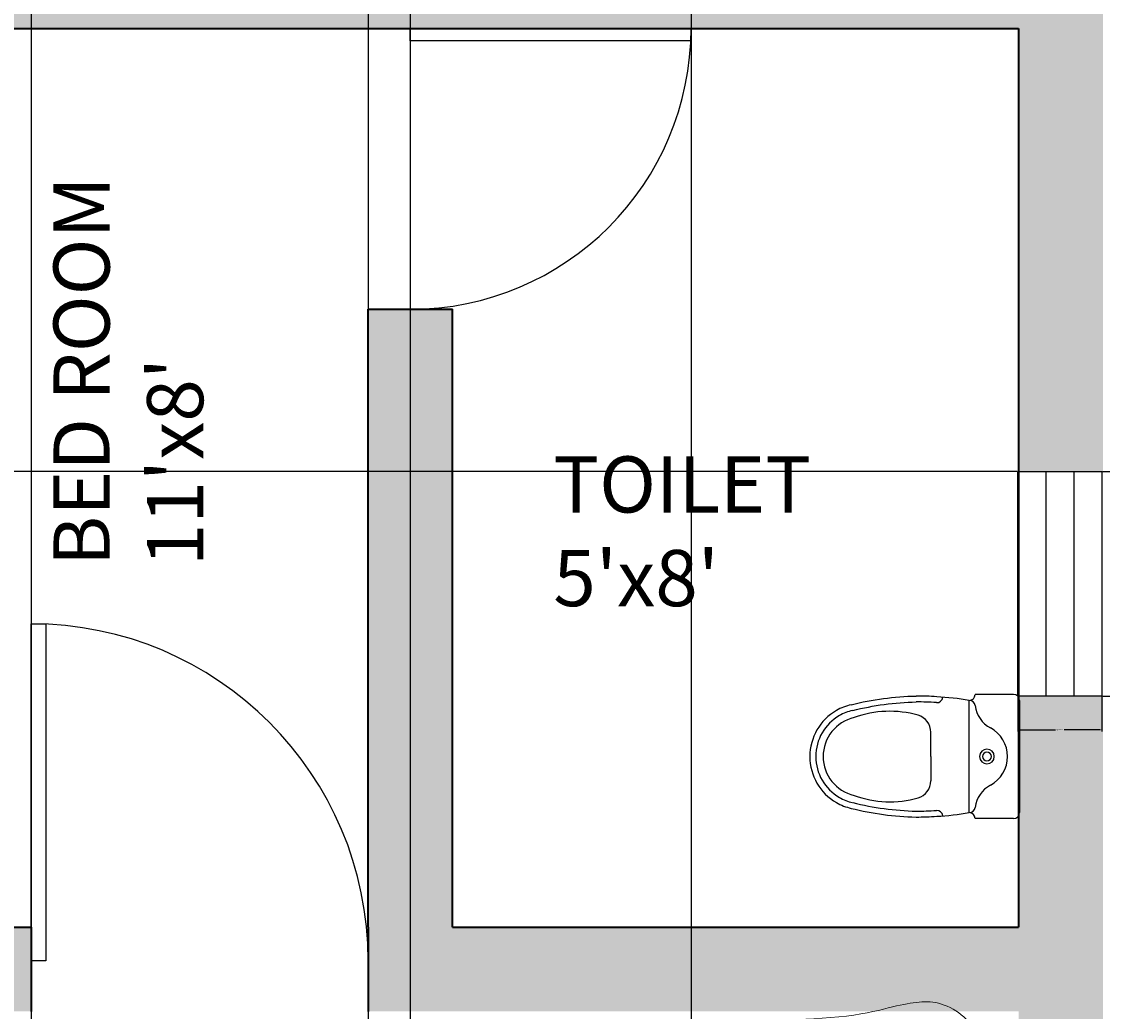
# Model space of a CAD drawing. Units: millimetres. Extents: x 2817 to 5038, y 1110 to 3565.
# Tile 8 of 21: x 2946 to 3061, y 1265 to 1371. Entities that reach past the tile are written whole.
import ezdxf

# ---------------------------------------------------------------- set-up
doc = ezdxf.new("R2010")
doc.units = ezdxf.units.MM
for name, color, linetype, lineweight in [('A-ANNO-DIMS', 2, 'Continuous', 18), ('A-AREA-IDEN', 7, 'Continuous', 18), ('A-FLOR-FIXT', 8, 'Continuous', 18), ('A-WALL', 7, 'Continuous', 35), ('DOOR&WINDOW', 1, 'Continuous', 25), ('FURNITURE', 219, 'Continuous', 18)]:
    doc.layers.add(name, color=color, linetype=linetype, lineweight=lineweight)
doc.layers.add('A-WALL-PATT', color=51, linetype='Continuous', lineweight=13, true_color=0xf7f281)
doc.layers.add('THIET-BI', color=21, linetype='Continuous')
doc.styles.get("Standard").update_dxf_attribs({"font": 'arial.ttf'})
doc.dimstyles.get("Standard").update_dxf_attribs({"dimtxt": 0.18, "dimasz": 0.18, "dimexe": 0.18, "dimexo": 0.0625, "dimgap": 0.09, "dimtad": 0, "dimtih": 1, "dimtoh": 1, "dimdec": 4, "dimzin": 0, "dimdsep": 46, "dimtxsty": 'Standard', "dimcen": 0.09, "dimadec": 0, "dimazin": 0, "dimtfac": 1, "dimtdec": 4, "dimtofl": 0, "dimtmove": 0, "dimatfit": 3, "dimfxl": 1, "dimtolj": 1, "dimtzin": 0, "dimarcsym": 0})

# ---------------------------------------------------------------- blocks, each defined once
blk = doc.blocks.new('*U2')
for p, q in [((0, 0), (0, -6)), ((40, 0), (40, -6))]:
    blk.add_line(p, q)
blk.add_lwpolyline([(0, 0), (0, 40), (1.75, 40), (1.75, 0)], close=True)
blk.add_arc((0, 0), 40, 0, 90)
blk = doc.blocks.new('A$C2E47758B')
for p, q in [((136.2, 1910.7), (127.9, 1907.3)), ((144.4, 1913.5), (136.2, 1910.7)), ((152.6, 1915.7), (144.4, 1913.5)), ((160.6, 1917.4), (152.6, 1915.7)), ((168.6, 1918.7), (160.6, 1917.4)), ((176.5, 1919.5), (168.6, 1918.7)), ((184.4, 1919.9), (176.5, 1919.5)), ((192.3, 1919.9), (184.4, 1919.9)), ((200.2, 1919.6), (192.3, 1919.9)), ((208.2, 1919.1), (200.2, 1919.6)), ((216.4, 1918.3), (208.2, 1919.1)), ((224.7, 1917.3), (216.4, 1918.3)), ((233.3, 1916), (224.7, 1917.3)), ((242.3, 1914.5), (233.3, 1916)), ((251.8, 1912.6), (242.3, 1914.5)), ((261.8, 1910.5), (251.8, 1912.6)), ((272.6, 1908.1), (261.8, 1910.5)), ((87.8, 1883), (80.6, 1876.8)), ((95.4, 1888.9), (87.8, 1883)), ((103.3, 1894.2), (95.4, 1888.9)), ((111.3, 1899.1), (103.3, 1894.2)), ((119.6, 1903.5), (111.3, 1899.1)), ((127.9, 1907.3), (119.6, 1903.5)), ((284, 1905.3), (272.6, 1908.1)), ((296.4, 1902.3), (284, 1905.3)), ((309.7, 1899), (296.4, 1902.3)), ((324, 1895.5), (309.7, 1899)), ((339.5, 1892), (324, 1895.5)), ((356.2, 1888.6), (339.5, 1892)), ((374.2, 1885.2), (356.2, 1888.6)), ((393.6, 1882.1), (374.2, 1885.2)), ((414.5, 1879.2), (393.6, 1882.1)), ((436.8, 1876.8), (414.5, 1879.2)), ((61.4, 1854.6), (55.6, 1845.5)), ((67.4, 1862.7), (61.4, 1854.6)), ((73.8, 1870), (67.4, 1862.7)), ((80.6, 1876.8), (73.8, 1870)), ((460.2, 1874.7), (436.8, 1876.8)), ((484, 1872.9), (460.2, 1874.7)), ((507.6, 1871.3), (484, 1872.9)), ((530.4, 1869.9), (507.6, 1871.3)), ((551.8, 1868.7), (530.4, 1869.9)), ((571.3, 1867.6), (551.8, 1868.7)), ((588.2, 1866.5), (571.3, 1867.6)), ((602.2, 1865.5), (588.2, 1866.5)), ((613.4, 1864.4), (602.2, 1865.5)), ((622.2, 1863.3), (613.4, 1864.4)), ((628.9, 1862.1), (622.2, 1863.3)), ((634, 1860.9), (628.9, 1862.1)), ((637.8, 1859.6), (634, 1860.9)), ((640.6, 1858.2), (637.8, 1859.6)), ((642.9, 1856.7), (640.6, 1858.2)), ((644.9, 1855), (642.9, 1856.7)), ((646.7, 1853.2), (644.9, 1855)), ((648.3, 1851.2), (646.7, 1853.2)), ((649.7, 1849), (648.3, 1851.2)), ((650.8, 1846.6), (649.7, 1849)), ((44.9, 1823.7), (39.9, 1810.7)), ((50.2, 1835.3), (44.9, 1823.7)), ((55.6, 1845.5), (50.2, 1835.3)), ((647.5, 1816.2), (650, 1821.2)), ((650, 1821.2), (651.7, 1825.8)), ((651.7, 1843.9), (650.8, 1846.6)), ((652.4, 1840.9), (651.7, 1843.9)), ((651.7, 1825.8), (652.5, 1830.1)), ((652.8, 1837.6), (652.4, 1840.9)), ((652.5, 1830.1), (652.9, 1834)), ((652.9, 1834), (652.8, 1837.6)), ((35, 1796), (30.2, 1779.2)), ((39.9, 1810.7), (35, 1796)), ((211.4, 1805.2), (169.1, 1786.1)), ((249.5, 1811.5), (211.4, 1805.2)), ((319.3, 1809.4), (249.5, 1811.5)), ((266.4, 1781), (629.3, 1800.3)), ((633, 1799.3), (319.3, 1809.4)), ((626.2, 1798.6), (626.2, 1799)), ((627, 1799), (626.2, 1798.6)), ((633, 1799.3), (639.1, 1805.3)), ((639.1, 1805.3), (643.9, 1810.9)), ((643.9, 1810.9), (647.5, 1816.2)), ((25.6, 1759.2), (21, 1734.4)), ((30.2, 1779.2), (25.6, 1759.2)), ((169.1, 1786.1), (133.2, 1748)), ((211.4, 1721.7), (232.6, 1757.7)), ((232.6, 1757.7), (266.4, 1781)), ((232.6, 1757.7), (266.4, 1781)), ((21, 1734.4), (16.6, 1703.5)), ((133.2, 1748), (103.5, 1682.4)), ((16.6, 1703.5), (12.3, 1665)), ((12.3, 1665), (8.1, 1617.5)), ((103.5, 1682.4), (84.5, 1595.6)), ((8.1, 1617.5), (4, 1559.6)), ((84.5, 1595.6), (78.2, 1536.4)), ((4, 1559.6), (0, 1489.8)), ((78.2, 1536.4), (78.2, 1489.8)), ((78.2, 1515.4), (78.2, 1493.9)), ((211.4, 1169.1), (232.6, 1215)), ((702.1, 1170.7), (702.1, 749.2)), ((181.8, 1046.7), (211.4, 1169.1)), ((173.3, 987.5), (181.8, 1046.7)), ((173.3, 985.3), (173.3, 987.5)), ((173.3, 932.4), (173.3, 985.3)), ((181.8, 873.2), (173.3, 932.4)), ((211.4, 758.9), (181.8, 873.2)), ((211.4, 757.7), (232.6, 721.7)), ((232.6, 721.7), (266.4, 681.7)), ((232.6, 637.5), (266.4, 681.7)), ((266.4, 681.7), (629.3, 680.2)), ((266.4, 681.7), (629.3, 680.2)), ((627, 680.1), (626.2, 679.6)), ((626.2, 679.6), (626.2, 680)), ((627, 679.2), (626.2, 679.6)), ((626.2, 679.6), (626.2, 679.2)), ((211.4, 601.6), (232.6, 637.5)), ((211.4, 601.6), (181.8, 487.3)), ((702.1, 189.8), (702.1, 611.2)), ((181.8, 487.3), (173.3, 428)), ((4, 360.3), (0, 430.1)), ((78.2, 383.5), (78.2, 410.9)), ((173.3, 430.1), (173.3, 373)), ((173.3, 428), (173.3, 430.1)), ((84.5, 324.3), (78.2, 383.5)), ((173.3, 373), (181.8, 313.7)), ((8.1, 302.4), (4, 360.3)), ((103.5, 237.5), (84.5, 324.3)), ((181.8, 313.7), (211.4, 199.4)), ((12.3, 254.9), (8.1, 302.4)), ((16.6, 216.4), (12.3, 254.9)), ((21, 185.5), (16.6, 216.4)), ((133.2, 171.9), (103.5, 237.5)), ((25.6, 160.7), (21, 185.5)), ((211.4, 199.4), (232.6, 163.4)), ((30.2, 140.7), (25.6, 160.7)), ((169.1, 133.8), (133.2, 171.9)), ((232.6, 163.4), (266.4, 140.1)), ((35, 123.9), (30.2, 140.7)), ((39.9, 109.2), (35, 123.9)), ((211.4, 114.7), (169.1, 133.8)), ((266.4, 140.1), (629.3, 120.7)), ((44.9, 96.2), (39.9, 109.2)), ((50.2, 84.6), (44.9, 96.2)), ((249.5, 108.4), (211.4, 114.7)), ((319.3, 110.5), (249.5, 108.4)), ((633, 120.7), (319.3, 110.5)), ((626.2, 121.3), (626.2, 120.9)), ((627, 120.9), (626.2, 121.3)), ((633, 120.7), (639.1, 114.6)), ((639.1, 114.6), (643.9, 109)), ((643.9, 109), (647.5, 103.7)), ((647.5, 103.7), (650, 98.7)), ((650, 98.7), (651.7, 94.1)), ((651.7, 94.1), (652.5, 89.8)), ((55.6, 74.4), (50.2, 84.6)), ((61.4, 65.3), (55.6, 74.4)), ((67.4, 57.2), (61.4, 65.3)), ((640.6, 61.7), (637.8, 60.3)), ((642.9, 63.2), (640.6, 61.7)), ((644.9, 64.9), (642.9, 63.2)), ((646.7, 66.7), (644.9, 64.9)), ((648.3, 68.7), (646.7, 66.7)), ((649.7, 70.9), (648.3, 68.7)), ((650.8, 73.3), (649.7, 70.9)), ((651.7, 76), (650.8, 73.3)), ((652.4, 79), (651.7, 76)), ((652.8, 82.3), (652.4, 79)), ((652.5, 89.8), (652.9, 85.9)), ((652.9, 85.9), (652.8, 82.3)), ((73.8, 49.9), (67.4, 57.2)), ((80.6, 43.1), (73.8, 49.9)), ((87.8, 36.9), (80.6, 43.1)), ((95.4, 31.1), (87.8, 36.9)), ((103.3, 25.7), (95.4, 31.1)), ((356.2, 31.4), (339.5, 27.9)), ((374.2, 34.7), (356.2, 31.4)), ((393.6, 37.8), (374.2, 34.7)), ((414.5, 40.7), (393.6, 37.8)), ((436.8, 43.1), (414.5, 40.7)), ((460.2, 45.2), (436.8, 43.1)), ((484, 47), (460.2, 45.2)), ((507.6, 48.6), (484, 47)), ((530.4, 50), (507.6, 48.6)), ((551.8, 51.2), (530.4, 50)), ((571.3, 52.3), (551.8, 51.2)), ((588.2, 53.4), (571.3, 52.3)), ((602.2, 54.4), (588.2, 53.4)), ((613.4, 55.5), (602.2, 54.4)), ((622.2, 56.6), (613.4, 55.5)), ((628.9, 57.8), (622.2, 56.6)), ((634, 59), (628.9, 57.8)), ((637.8, 60.3), (634, 59)), ((111.3, 20.8), (103.3, 25.7)), ((119.6, 16.4), (111.3, 20.8)), ((127.9, 12.6), (119.6, 16.4)), ((136.2, 9.2), (127.9, 12.6)), ((144.4, 6.4), (136.2, 9.2)), ((152.6, 4.2), (144.4, 6.4)), ((160.6, 2.5), (152.6, 4.2)), ((168.6, 1.3), (160.6, 2.5)), ((176.5, 0.5), (168.6, 1.3)), ((184.4, 0), (176.5, 0.5)), ((192.3, 0), (184.4, 0)), ((200.2, 0.3), (192.3, 0)), ((208.2, 0.8), (200.2, 0.3)), ((216.4, 1.6), (208.2, 0.8)), ((224.7, 2.6), (216.4, 1.6)), ((233.3, 3.9), (224.7, 2.6)), ((242.3, 5.4), (233.3, 3.9)), ((251.8, 7.3), (242.3, 5.4)), ((261.8, 9.4), (251.8, 7.3)), ((272.6, 11.8), (261.8, 9.4)), ((284, 14.6), (272.6, 11.8)), ((296.4, 17.6), (284, 14.6)), ((309.7, 20.9), (296.4, 17.6)), ((324, 24.4), (309.7, 20.9)), ((339.5, 27.9), (324, 24.4))]:
    blk.add_line(p, q)
for points in [[(629.3, 1239.7), (266.4, 1238.2), (629.3, 1239.7, 0.429937), (702.1, 1308.7), (702.1, 1730.1, 0.429937), (629.3, 1799.2)], [(78.2, 410.9, -0.050936), (78.2, 1525.6, 12.167348)], [(0, 430.1, -0.05358), (0, 1489.8, 12.163767)], [(173.3, 1494, 0.004989), (173.3, 401.5, 0.847003)]]:
    blk.add_lwpolyline(points, format="xyb")
blk.add_lwpolyline([(211.4, 1720.5), (181.8, 1606.2), (173.3, 1546.9), (173.3, 1494), (173.3, 1491.9), (181.8, 1432.6), (211.4, 1304.3), (232.6, 1261.5), (266.4, 1238.2), (232.6, 1215)])
for centre, start, end in [((633, 1170.7), 0, 93.0587), ((633, 749.2), 266.9413, 360), ((633, 749.2), 266.9413, 360), ((633, 611.2), 0, 93.0587), ((633, 611.2), 0, 93.0587), ((633, 611.2), 0, 93.0587), ((633, 189.8), 266.9413, 360)]:
    blk.add_arc(centre, 69.1, start, end)
blk = doc.blocks.new('A$C7C314EA1')
at = {"layer": 'THIET-BI'}
for p, q in [((20, 420), (150, 420)), ((0, 20), (0, 400)), ((170, 400), (170, 20)), ((300, 210), (300, 292.2)), ((300, 210), (300, 127.8)), ((20, 0), (150, 0)), ((20, 0), (150, 0))]:
    blk.add_line(p, q, dxfattribs=at)
for points in [[(279.9, 412.5, 0.02753), (170, 400, 0.02753)], [(569.7, 385.6, 0.054905), (350, 415, 0.054905)], [(564.9, 366.1, 0.054905), (349.5, 395, 0.054905)], [(300, 210), (300, 290, 0.704392)], [(300, 210), (300, 130, -0.704392)], [(564.9, 53.9, -0.054905), (349.5, 25, -0.054905)], [(170, 20, 0.02753), (279.9, 7.5, 0.02753)], [(569.7, 34.4, -0.054905), (350, 5, -0.054905)]]:
    blk.add_lwpolyline(points, format="xyb", dxfattribs=at)
for centre, radius, start, end in [((20, 400), 20, 90, 180), ((170, 420), 20, 180, 270), ((279.9, 412.5), 20, 184.5905, 273.8823), ((350, -585), 1000, 90, 94.0204), ((51, 395.2), 100, 298.1382, 352.7323), ((170, 380), 20, 90, 172.7323), ((350, -585), 980, 90, 94.0204), ((530, 210), 180, 60, 77.2425), ((360, 292.2), 60, 105.9249, 180), ((439, 15.2), 348.1, 69.701, 105.9249), ((530, 210), 135, 0, 77.2425), ((530, 210), 160, 60, 77.2425), ((530, 210), 160, 0, 60), ((530, 210), 180, 0, 60), ((150, 210), 110, 118.1382, 180), ((110, 210), 25, 0, 180), ((110, 210), 25, 0, 180), ((110, 210), 15, 0, 180), ((110, 210), 15, 0, 180), ((150, 210), 110, 180, 241.8618), ((150, 210), 110, 180, 241.8618), ((110, 210), 25, 180, 0), ((110, 210), 25, 180, 0), ((110, 210), 15, 180, 0), ((110, 210), 15, 180, 0), ((530, 210), 135, 282.7575, 0), ((530, 210), 160, 300, 0), ((530, 210), 180, 300, 0), ((51, 24.8), 100, 7.2677, 61.8618), ((51, 24.8), 100, 7.2677, 61.8618), ((360, 127.8), 60, 180, 254.0751), ((439, 404.8), 348.1, 254.0751, 290.299), ((170, 40), 20, 187.2677, 270), ((170, 40), 20, 187.2677, 270), ((530, 210), 160, 282.7575, 300), ((530, 210), 180, 282.7575, 300), ((20, 20), 20, 180, 270), ((170, 0), 20, 90, 180), ((279.9, 7.5), 20, 86.1177, 175.4095), ((350, 1005), 1000, 265.9796, 270), ((350, 1005), 980, 265.9796, 270)]:
    blk.add_arc(centre, radius, start, end, dxfattribs=at)
blk = doc.blocks.new('WIN-2FT')
for p, q in [((0, 24), (9, 24)), ((0, 0), (0, 24)), ((3, 24), (3, 0)), ((6, 24), (6, 0)), ((9, 24), (9, 0)), ((9, 0), (0, 0))]:
    blk.add_line(p, q)
blk = doc.blocks.new('*D16')
at = {"layer": 'A-ANNO-DIMS', "color": 0, "lineweight": -2, "transparency": 16777216}
for p, q in [((3061.2, 1323.1), (3064.92, 1323.1)), ((3064.74, 1322.92), (3064.74, 1311.28)), ((3064.74, 1299.28), (3064.74, 1310.92)), ((3061.2, 1299.1), (3064.92, 1299.1))]:
    blk.add_line(p, q, dxfattribs=at)
for points in [[(3064.71, 1322.92), (3064.77, 1322.92), (3064.74, 1323.1)], [(3064.71, 1299.28), (3064.77, 1299.28), (3064.74, 1299.1)]]:
    blk.add_solid(points, dxfattribs=at)
at = {"layer": 'Defpoints', "color": 0, "lineweight": -2, "transparency": 16777216}
for p in [(3061.14, 1323.1), (3064.74, 1323.1), (3061.14, 1299.1)]:
    blk.add_point(p, dxfattribs=at)
at = {"layer": 'A-ANNO-DIMS', "color": 0, "transparency": 16777216, "insert": (3064.74, 1311.1), "char_height": 0.18, "attachment_point": 5}
blk.add_mtext('\\A1;WIN. 24 TYP.', dxfattribs=at)
blk = doc.blocks.new('*D17')
at = {"layer": 'A-ANNO-DIMS', "color": 0, "lineweight": -2, "transparency": 16777216}
for p, q in [((3052.14, 1299.04), (3052.14, 1295.32)), ((3061.14, 1299.04), (3061.14, 1295.32)), ((3052.32, 1295.5), (3056.18, 1295.5)), ((3060.96, 1295.5), (3057.1, 1295.5))]:
    blk.add_line(p, q, dxfattribs=at)
for points in [[(3052.32, 1295.53), (3052.32, 1295.47), (3052.14, 1295.5)], [(3060.96, 1295.53), (3060.96, 1295.47), (3061.14, 1295.5)]]:
    blk.add_solid(points, dxfattribs=at)
at = {"layer": 'Defpoints', "color": 0, "lineweight": -2, "transparency": 16777216}
for p in [(3052.14, 1299.1), (3061.14, 1299.1), (3061.14, 1295.5)]:
    blk.add_point(p, dxfattribs=at)
at = {"layer": 'A-ANNO-DIMS', "color": 0, "transparency": 16777216, "insert": (3056.64, 1295.5), "char_height": 0.18, "attachment_point": 5}
blk.add_mtext('\\A1;9 TYP.', dxfattribs=at)
blk = doc.blocks.new('*D34')
at = {"layer": 'A-ANNO-DIMS', "color": 0, "lineweight": -2, "transparency": 16777216}
for p, q in [((2946.74, 1500.37), (2946.74, 1110.01)), ((2982.74, 1500.37), (2982.74, 1110.01)), ((2946.92, 1110.19), (2964.52, 1110.19)), ((2982.56, 1110.19), (2964.96, 1110.19))]:
    blk.add_line(p, q, dxfattribs=at)
for points in [[(2946.92, 1110.22), (2946.92, 1110.16), (2946.74, 1110.19)], [(2982.56, 1110.22), (2982.56, 1110.16), (2982.74, 1110.19)]]:
    blk.add_solid(points, dxfattribs=at)
at = {"layer": 'Defpoints', "color": 0, "lineweight": -2, "transparency": 16777216}
for p in [(2946.74, 1500.44), (2982.74, 1500.44), (2982.74, 1110.19)]:
    blk.add_point(p, dxfattribs=at)
at = {"layer": 'A-ANNO-DIMS', "color": 0, "transparency": 16777216, "insert": (2964.74, 1110.19), "char_height": 0.18, "attachment_point": 5}
blk.add_mtext('\\A1;36', dxfattribs=at)
blk = doc.blocks.new('*D35')
at = {"layer": 'A-ANNO-DIMS', "color": 0, "lineweight": -2, "transparency": 16777216}
for p, q in [((2987.24, 1605.37), (2987.24, 1110.01)), ((3017.24, 1605.37), (3017.24, 1110.01)), ((2987.42, 1110.19), (3002.02, 1110.19)), ((3017.06, 1110.19), (3002.46, 1110.19))]:
    blk.add_line(p, q, dxfattribs=at)
for points in [[(2987.42, 1110.22), (2987.42, 1110.16), (2987.24, 1110.19)], [(3017.06, 1110.22), (3017.06, 1110.16), (3017.24, 1110.19)]]:
    blk.add_solid(points, dxfattribs=at)
at = {"layer": 'Defpoints', "color": 0, "lineweight": -2, "transparency": 16777216}
for p in [(2987.24, 1605.44), (3017.24, 1605.44), (3017.24, 1110.19)]:
    blk.add_point(p, dxfattribs=at)
at = {"layer": 'A-ANNO-DIMS', "color": 0, "transparency": 16777216, "insert": (3002.24, 1110.19), "char_height": 0.18, "attachment_point": 5}
blk.add_mtext('\\A1;30', dxfattribs=at)
blk = doc.blocks.new('*D47')
at = {"layer": 'A-ANNO-DIMS', "color": 0, "lineweight": -2, "transparency": 16777216}
for p, q in [((3052.18, 1370.44), (2817.31, 1370.44)), ((2817.49, 1370.26), (2817.49, 1346.95)), ((2817.49, 1323.28), (2817.49, 1346.58)), ((3052.08, 1323.1), (2817.31, 1323.1))]:
    blk.add_line(p, q, dxfattribs=at)
for points in [[(2817.46, 1370.26), (2817.52, 1370.26), (2817.49, 1370.44)], [(2817.46, 1323.28), (2817.52, 1323.28), (2817.49, 1323.1)]]:
    blk.add_solid(points, dxfattribs=at)
at = {"layer": 'Defpoints', "color": 0, "lineweight": -2, "transparency": 16777216}
for p in [(2817.49, 1370.44), (3052.24, 1370.44), (3052.14, 1323.1)]:
    blk.add_point(p, dxfattribs=at)
at = {"layer": 'A-ANNO-DIMS', "color": 0, "transparency": 16777216, "insert": (2817.49, 1346.77), "char_height": 0.18, "attachment_point": 5}
blk.add_mtext('\\A1;47.34', dxfattribs=at)

msp = doc.modelspace()

# ---------------------------------------------------------------- hatches: boundary and pattern name
at = {"layer": 'A-WALL-PATT'}
h = msp.add_hatch(color=256, dxfattribs=at)
h.dxf.hatch_style = 1
h.paths.add_polyline_path([(3186.7393, 1614.4357), (2841.7393, 1614.4357), (2841.7393, 1568.614), (2850.7393, 1568.7609), (2850.7393, 1605.4357), (2982.7393, 1605.4357), (2991.7393, 1605.4357), (3052.2393, 1605.4357), (3052.2393, 1573.7835), (3061.2393, 1573.7835), (3061.2393, 1605.4357), (3182.2393, 1605.4357), (3182.2393, 1143.4357), (3181.2393, 1143.4357), (3181.2393, 1134.4357), (3186.7393, 1134.4357)])
h.paths.add_polyline_path([(3061.2393, 1143.4357), (3061.2393, 1147.4357), (3052.2393, 1147.4357), (3052.2393, 1143.4357), (2850.7393, 1143.4357), (2850.7393, 1145.2996), (2841.7393, 1145.2996), (2841.7393, 1134.4357), (3061.2393, 1134.4357)], flags=17)
h.paths.add_polyline_path([(2850.7393, 1265.4357), (2946.7393, 1265.4357), (2946.7393, 1270.8357), (2946.7393, 1274.4357), (2850.7393, 1274.4357), (2850.7381, 1274.4357), (2850.7381, 1274.2564), (2841.7393, 1274.2564), (2841.7393, 1193.1527), (2850.7393, 1193.2996)], flags=17)
h.paths.add_polyline_path([(3061.2393, 1299.098), (3052.2393, 1299.098), (3052.2393, 1274.4357), (2991.7393, 1274.4357), (2991.7393, 1340.4357), (2982.7393, 1340.4357), (2982.7393, 1274.4357), (2982.7393, 1265.4357), (3052.2393, 1265.4357), (3052.2393, 1259.143), (3061.2393, 1259.2899)], flags=17)
h.paths.add_polyline_path([(3061.2393, 1383.4357), (3052.2393, 1383.4357), (3052.2393, 1379.4357), (2931.7393, 1379.4357), (2922.7393, 1379.4357), (2850.7393, 1379.4357), (2850.7381, 1379.4357), (2850.7381, 1379.3646), (2841.7393, 1379.3646), (2841.7393, 1322.1095), (2850.7393, 1322.2564), (2850.7393, 1370.4357), (2982.7393, 1370.4357), (2987.2393, 1370.4357), (3017.2393, 1370.4357), (3052.2393, 1370.4357), (3052.2393, 1323.098), (3061.2393, 1323.098)], flags=17)

# ---------------------------------------------------------------- linework, layer by layer
at = {"layer": 'A-WALL'}
for p, q in [((2850.7393, 1370.4357), (2982.7393, 1370.4357)), ((2982.7393, 1370.4357), (2991.7393, 1370.4357)), ((2991.7393, 1370.4357), (3052.2393, 1370.4357)), ((3052.2393, 1370.4357), (3052.2393, 1274.4357)), ((2982.7393, 1274.4357), (2982.7393, 1340.4357)), ((2982.7393, 1340.4357), (2991.7393, 1340.4357)), ((2991.7393, 1274.4357), (2991.7393, 1340.4357)), ((2850.7393, 1274.4357), (2946.7393, 1274.4357)), ((2946.7393, 1274.4357), (2946.7393, 1265.4357)), ((2982.7393, 1274.4357), (2982.7393, 1265.4357)), ((2991.7393, 1274.4357), (3052.2393, 1274.4357))]:
    msp.add_line(p, q, dxfattribs=at)

# ---------------------------------------------------------------- block references
at = {"layer": 'A-FLOR-FIXT', "xscale": 0.0315352998736587, "yscale": 0.0315352998736587, "zscale": 0.0315352998736587, "rotation": 180}
msp.add_blockref('A$C7C314EA1', (3052.3225, 1299.2827), dxfattribs=at)
at = {"layer": 'DOOR&WINDOW', "xscale": 0.75, "yscale": 0.75, "zscale": 0.75, "rotation": 270}
msp.add_blockref('*U2', (2987.2393, 1370.4357), dxfattribs=at)
at = {"layer": 'DOOR&WINDOW'}
msp.add_blockref('WIN-2FT', (3052.1378, 1299.098), dxfattribs=at)
at = {"layer": 'DOOR&WINDOW', "xscale": 0.9, "yscale": 0.9, "zscale": 0.9}
msp.add_blockref('*U2', (2946.7393, 1270.8357), dxfattribs=at)
at = {"layer": 'FURNITURE', "xscale": -0.0374923371980192, "yscale": 0.0374923371980192, "zscale": 0.0374923371980192}
msp.add_blockref('A$C2E47758B', (3049.4066, 1194.48), dxfattribs=at)

# ---------------------------------------------------------------- texts
at = {"layer": 'A-AREA-IDEN', "insert": (2949.1185, 1312.9909), "char_height": 6, "attachment_point": 1, "rotation": 90}
msp.add_mtext_dynamic_manual_height_columns("BED ROOM\\P11'x8'", width=51.672891, gutter_width=12.5, heights=[0], dxfattribs=at)
at = {"layer": 'A-AREA-IDEN', "insert": (3002.5229, 1324.7239), "char_height": 6, "attachment_point": 1}
msp.add_mtext_dynamic_manual_height_columns("TOILET\\P5'x8'", width=42.068425, gutter_width=12.5, heights=[0], dxfattribs=at)

# ---------------------------------------------------------------- dimensions: what is measured, and where the dimension line sits
at = {"layer": 'A-ANNO-DIMS'}
for base, p1, p2, picture, middle in [((3017.2393, 1110.1857), (2987.2393, 1605.4357), (3017.2393, 1605.4357), '*D35', (3002.2393, 1110.1857)), ((2982.7393, 1110.1857), (2946.7393, 1500.4357), (2982.7393, 1500.4357), '*D34', (2964.7393, 1110.1857))]:
    dim = msp.add_linear_dim(base=base, p1=p1, p2=p2, dimstyle='Standard', override={"dimdec": 0, "dimlfac": 1, "dimrnd": 0, "dimzin": 0, "dimdsep": 46, "dimlunit": 2}, dxfattribs=at)
    dim.commit()
    dim.dimension.update_dxf_attribs({"geometry": picture, "text_midpoint": middle})
dim = msp.add_linear_dim(base=(2817.4881, 1370.4357), p1=(3052.1378, 1323.098), p2=(3052.2393, 1370.4357), angle=90, dimstyle='Standard', override={"dimdec": 2, "dimlfac": 1, "dimrnd": 0, "dimzin": 0, "dimdsep": 46, "dimlunit": 2}, dxfattribs=at)
dim.commit()
dim.dimension.update_dxf_attribs({"geometry": '*D47', "text_midpoint": (2817.4881, 1346.7669)})
dim = msp.add_linear_dim(base=(3064.7378, 1323.098), p1=(3061.1378, 1299.098), p2=(3061.1378, 1323.098), angle=90, text='WIN. <> TYP.', dimstyle='Standard', override={"dimdec": 0, "dimlfac": 1, "dimrnd": 0, "dimzin": 0, "dimdsep": 46, "dimlunit": 2}, dxfattribs=at)
dim.commit()
dim.dimension.update_dxf_attribs({"geometry": '*D16', "text_midpoint": (3064.7378, 1311.098)})
dim = msp.add_linear_dim(base=(3061.1378, 1295.498), p1=(3052.1378, 1299.098), p2=(3061.1378, 1299.098), text='<> TYP.', dimstyle='Standard', override={"dimdec": 0, "dimlfac": 1, "dimrnd": 0, "dimzin": 0, "dimdsep": 46, "dimlunit": 2}, dxfattribs=at)
dim.commit()
dim.dimension.update_dxf_attribs({"geometry": '*D17', "text_midpoint": (3056.6378, 1295.498)})

doc.saveas('drawing.dxf')
